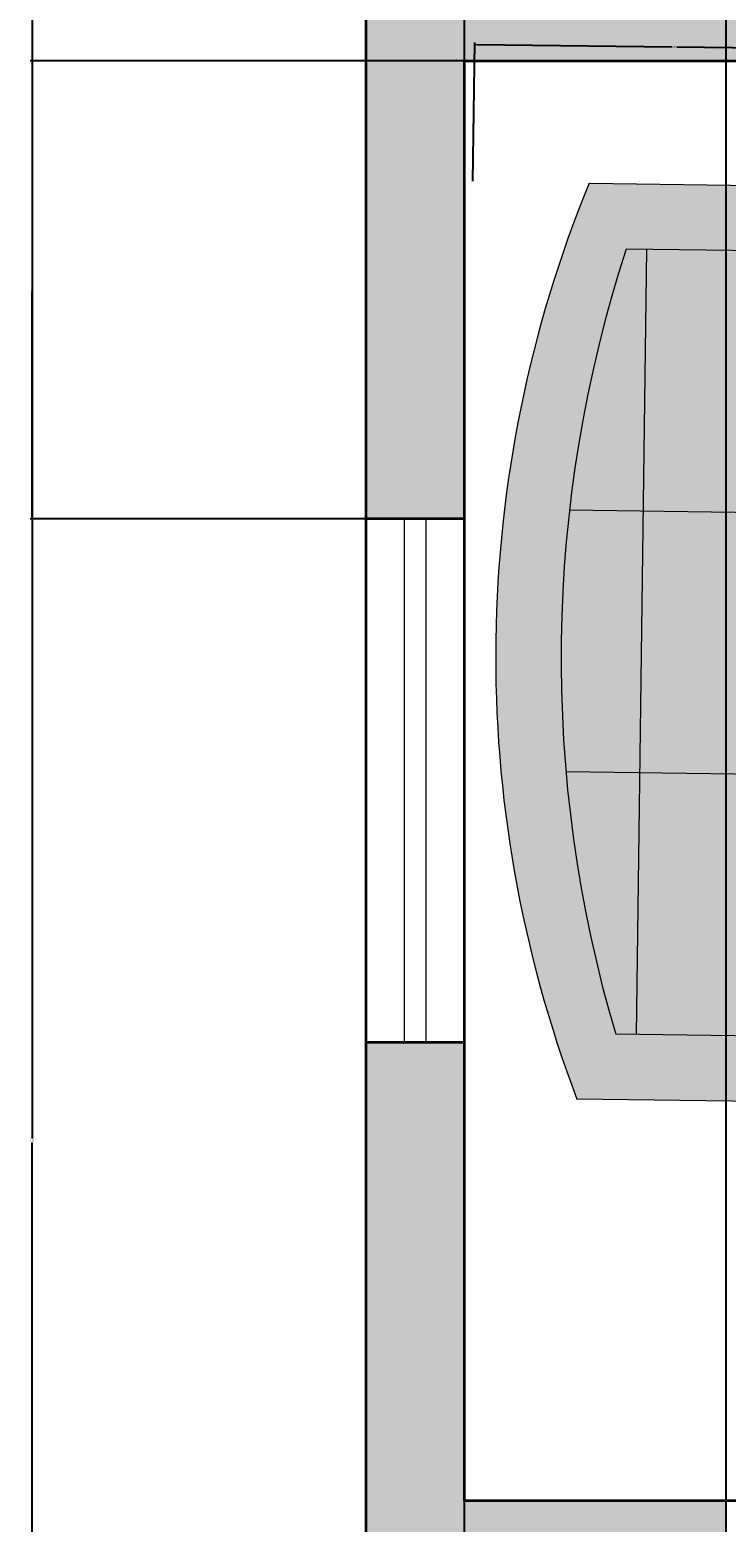
# Model space of a CAD drawing. Units: inches. Extents: x 1567 to 1964, y 1813 to 2447.
# Tile 7 of 28: x 1567 to 1630, y 2125 to 2262. Entities that reach past the tile are written whole.
import ezdxf

# ---------------------------------------------------------------- set-up
doc = ezdxf.new("R2010")
doc.units = ezdxf.units.IN
for name, color, linetype, lineweight in [('A-ANNO-DIMS', 2, 'Continuous', 18), ('A-FURN', 8, 'Continuous', 18), ('A-GLAZ', 4, 'Continuous', 18), ('A-WALL', 7, 'Continuous', 35)]:
    doc.layers.add(name, color=color, linetype=linetype, lineweight=lineweight)
doc.layers.add('A-FURN-PATT', color=252, linetype='Continuous', lineweight=13, true_color=0x939598)
doc.layers.add('A-WALL-PATT', color=251, linetype='Continuous', lineweight=13, true_color=0x636466)
doc.styles.get("Standard").update_dxf_attribs({"font": 'arial.ttf'})
doc.dimstyles.get("Standard").update_dxf_attribs({"dimtxt": 0.18, "dimasz": 0.18, "dimexe": 0.18, "dimexo": 0.0625, "dimgap": 0.09, "dimtad": 0, "dimtih": 1, "dimtoh": 1, "dimdec": 4, "dimzin": 0, "dimdsep": 46, "dimtxsty": 'Standard', "dimcen": 0.09, "dimadec": 0, "dimazin": 0, "dimtfac": 1, "dimtdec": 4, "dimtofl": 0, "dimtmove": 0, "dimatfit": 3, "dimfxl": 1, "dimtolj": 1, "dimtzin": 0, "dimarcsym": 0})

# ---------------------------------------------------------------- blocks, each defined once
blk = doc.blocks.new('Sofa - Roundback 7 ft.')
for p, q in [((-12.00002, -32.4421), (-12.00003, -6.5971)), ((11.99997, -32.4421), (11.99998, -6.5971)), ((-36.000027, -34), (-36.000027, -11.4696)), ((35.99998, -34), (35.99998, -11.4696)), ((-35.999844, -13.3819), (35.9998, -13.3819)), ((-36.000027, -32.4421), (35.99998, -32.4421))]:
    blk.add_line(p, q)
for points in [[(-36.000027, -34), (-42.000027, -34), (-42.000027, -8)], [(41.99998, -8), (41.99998, -34), (35.99998, -34)]]:
    blk.add_lwpolyline(points)
for centre, radius, start, end in [((0, -114.25), 114.25, 68.43141, 111.5686), ((-0.00001, -127.1968), 121.1968, 72.72033, 107.2797)]:
    blk.add_arc(centre, radius, start, end)
blk = doc.blocks.new('WINDOW-48IN')
for p, q in [((0, 2), (48, 2)), ((0, 0), (48, 0))]:
    blk.add_line(p, q)
blk = doc.blocks.new('*D24')
at = {"layer": 'A-ANNO-DIMS', "color": 0, "lineweight": -2, "transparency": 16777216}
for p, q in [((1607.2, 2248.27), (1607.37, 2260.99)), ((1607.54, 2260.81), (1625.48, 2260.57)), ((1643.85, 2260.32), (1625.92, 2260.56)), ((1643.86, 2247.79), (1644.03, 2260.5))]:
    blk.add_line(p, q, dxfattribs=at)
at = {"layer": 'A-ANNO-DIMS', "color": 0, "transparency": 16777216}
for points in [[(1607.54, 2260.84), (1607.54, 2260.78), (1607.36, 2260.81)], [(1643.85, 2260.35), (1643.85, 2260.29), (1644.03, 2260.32)]]:
    blk.add_solid(points, dxfattribs=at)
at = {"layer": 'Defpoints', "color": 0, "transparency": 16777216}
for p in [(1607.36, 2260.81), (1607.2, 2248.21), (1643.86, 2247.72)]:
    blk.add_point(p, dxfattribs=at)
at = {"layer": 'A-ANNO-DIMS', "color": 0, "transparency": 16777216, "insert": (1625.7, 2260.57), "char_height": 0.18, "attachment_point": 5}
blk.add_mtext('\\A1;37', dxfattribs=at)
blk = doc.blocks.new('*D41')
at = {"layer": 'A-ANNO-DIMS', "color": 0, "lineweight": -2, "transparency": 16777216}
for p, q in [((1597.37, 2416.29), (1566.6, 2416.29)), ((1566.78, 2416.11), (1566.78, 2160.47)), ((1566.78, 1904.47), (1566.78, 2160.11)), ((1601.37, 1904.29), (1566.6, 1904.29))]:
    blk.add_line(p, q, dxfattribs=at)
at = {"layer": 'A-ANNO-DIMS', "color": 0, "transparency": 16777216}
for points in [[(1566.75, 2416.11), (1566.81, 2416.11), (1566.78, 2416.29)], [(1566.75, 1904.47), (1566.81, 1904.47), (1566.78, 1904.29)]]:
    blk.add_solid(points, dxfattribs=at)
at = {"layer": 'Defpoints', "color": 0, "transparency": 16777216}
for p in [(1566.78, 2416.29), (1597.43, 2416.29), (1601.43, 1904.29)]:
    blk.add_point(p, dxfattribs=at)
at = {"layer": 'A-ANNO-DIMS', "color": 0, "transparency": 16777216, "insert": (1566.78, 2160.29), "char_height": 0.18, "attachment_point": 5}
blk.add_mtext('\\A1;512', dxfattribs=at)
blk = doc.blocks.new('*D50')
at = {"layer": 'A-ANNO-DIMS', "color": 0, "lineweight": -2, "transparency": 16777216}
for p, q in [((1606.37, 2259.29), (1566.6, 2259.29)), ((1566.78, 2259.11), (1566.78, 2238.47)), ((1566.78, 2217.47), (1566.78, 2238.11)), ((1597.37, 2217.29), (1566.6, 2217.29))]:
    blk.add_line(p, q, dxfattribs=at)
at = {"layer": 'A-ANNO-DIMS', "color": 0, "transparency": 16777216}
for points in [[(1566.75, 2259.11), (1566.81, 2259.11), (1566.78, 2259.29)], [(1566.75, 2217.47), (1566.81, 2217.47), (1566.78, 2217.29)]]:
    blk.add_solid(points, dxfattribs=at)
at = {"layer": 'Defpoints', "color": 0, "transparency": 16777216}
for p in [(1606.43, 2259.29), (1566.78, 2217.29), (1597.43, 2217.29)]:
    blk.add_point(p, dxfattribs=at)
at = {"layer": 'A-ANNO-DIMS', "color": 0, "transparency": 16777216, "insert": (1566.78, 2238.29), "char_height": 0.18, "attachment_point": 5}
blk.add_mtext('\\A1;42', dxfattribs=at)
blk = doc.blocks.new('*D53')
at = {"layer": 'A-ANNO-DIMS', "color": 0, "lineweight": -2, "transparency": 16777216}
for p, q in [((1606.43, 1913.35), (1606.43, 2447.12)), ((1606.61, 2446.94), (1618.21, 2446.94)), ((1630.25, 2446.94), (1618.65, 2446.94)), ((1630.43, 1913.35), (1630.43, 2447.12))]:
    blk.add_line(p, q, dxfattribs=at)
at = {"layer": 'A-ANNO-DIMS', "color": 0, "transparency": 16777216}
for points in [[(1606.61, 2446.97), (1606.61, 2446.91), (1606.43, 2446.94)], [(1630.25, 2446.97), (1630.25, 2446.91), (1630.43, 2446.94)]]:
    blk.add_solid(points, dxfattribs=at)
at = {"layer": 'Defpoints', "color": 0, "transparency": 16777216}
for p in [(1630.43, 2446.94), (1606.43, 1913.29), (1630.43, 1913.29)]:
    blk.add_point(p, dxfattribs=at)
at = {"layer": 'A-ANNO-DIMS', "color": 0, "transparency": 16777216, "insert": (1618.43, 2446.94), "char_height": 0.18, "attachment_point": 5}
blk.add_mtext('\\A1;24', dxfattribs=at)
blk = doc.blocks.new('*D56')
at = {"layer": 'A-ANNO-DIMS', "color": 0, "lineweight": -2, "transparency": 16777216}
for p, q in [((1606.43, 2127.35), (1606.43, 2447.12)), ((1606.61, 2446.94), (1618.21, 2446.94)), ((1630.25, 2446.94), (1618.65, 2446.94)), ((1630.43, 2127.35), (1630.43, 2447.12))]:
    blk.add_line(p, q, dxfattribs=at)
at = {"layer": 'A-ANNO-DIMS', "color": 0, "transparency": 16777216}
for points in [[(1606.61, 2446.97), (1606.61, 2446.91), (1606.43, 2446.94)], [(1630.25, 2446.97), (1630.25, 2446.91), (1630.43, 2446.94)]]:
    blk.add_solid(points, dxfattribs=at)
at = {"layer": 'Defpoints', "color": 0, "transparency": 16777216}
for p in [(1630.43, 2446.94), (1606.43, 2127.29), (1630.43, 2127.29)]:
    blk.add_point(p, dxfattribs=at)
at = {"layer": 'A-ANNO-DIMS', "color": 0, "transparency": 16777216, "insert": (1618.43, 2446.94), "char_height": 0.18, "attachment_point": 5}
blk.add_mtext('\\A1;24', dxfattribs=at)
blk = doc.blocks.new('*D57')
at = {"layer": 'A-ANNO-DIMS', "color": 0, "lineweight": -2, "transparency": 16777216}
for p, q in [((1630.43, 2127.35), (1630.43, 2447.12)), ((1630.61, 2446.94), (1654.21, 2446.94)), ((1678.25, 2446.94), (1654.65, 2446.94)), ((1678.43, 2127.35), (1678.43, 2447.12))]:
    blk.add_line(p, q, dxfattribs=at)
at = {"layer": 'A-ANNO-DIMS', "color": 0, "transparency": 16777216}
for points in [[(1630.61, 2446.97), (1630.61, 2446.91), (1630.43, 2446.94)], [(1678.25, 2446.97), (1678.25, 2446.91), (1678.43, 2446.94)]]:
    blk.add_solid(points, dxfattribs=at)
at = {"layer": 'Defpoints', "color": 0, "transparency": 16777216}
for p in [(1678.43, 2446.94), (1630.43, 2127.29), (1678.43, 2127.29)]:
    blk.add_point(p, dxfattribs=at)
at = {"layer": 'A-ANNO-DIMS', "color": 0, "transparency": 16777216, "insert": (1654.43, 2446.94), "char_height": 0.18, "attachment_point": 5}
blk.add_mtext('\\A1;48', dxfattribs=at)

msp = doc.modelspace()

# ---------------------------------------------------------------- hatches: boundary and pattern name
at = {"layer": 'A-FURN-PATT'}
h = msp.add_hatch(color=256, dxfattribs=at)
h.dxf.hatch_style = 1
h.paths.add_polyline_path([(1621.2532, 2242.0229), (1643.7811, 2241.7239), (1643.8607, 2247.7234), (1617.863, 2248.0685, 0.19047621), (1616.7481, 2164.0759), (1642.7458, 2163.7308), (1642.8254, 2169.7302), (1620.2975, 2170.0293, -0.15194781)])
h.paths.add_polyline_path([(1673.5306, 2249.6607), (1653.8509, 2249.6607), (1653.8509, 2248.5031, 0.11764706), (1673.5306, 2248.5031)])
h.paths.add_polyline_path([(1706.0889, 2249.6607), (1686.4092, 2249.6607), (1686.4092, 2248.5031, 0.11764706), (1706.0889, 2248.5031)])
h.paths.add_polyline_path([(1782.4511, 2227.4197), (1766.4511, 2227.4197), (1766.2949, 2226.4197), (1782.6074, 2226.4197)])
h.paths.add_polyline_path([(1810.4511, 2227.4197), (1794.4511, 2227.4197), (1794.2949, 2226.4197), (1810.6074, 2226.4197)])
h.paths.add_polyline_path([(1743.9511, 2208.076), (1742.9511, 2207.9197), (1742.9511, 2191.9197), (1743.9511, 2191.7635)])
h.paths.add_polyline_path([(1782.6074, 2173.4197), (1766.2949, 2173.4197), (1766.4511, 2172.4197), (1782.4511, 2172.4197)])
h.paths.add_polyline_path([(1810.6074, 2173.4197), (1794.2949, 2173.4197), (1794.4511, 2172.4197), (1810.4511, 2172.4197)])
h.paths.add_polyline_path([(1861.053, 2006.5071), (1845.8531, 2006.5071), (1861.053, 1991.3071)])
h.paths.add_polyline_path([(1905.853, 1993.7071), (1861.053, 1993.7071), (1861.053, 1991.3071), (1905.853, 1991.3071)])
h.paths.add_polyline_path([(1919.7245, 2257.29, 0.50000012), (1918.7245, 2258.29), (1901.7245, 2258.29, 0.50000012), (1900.7245, 2257.29), (1900.7245, 2253.29, 0.50000012), (1901.7245, 2252.29), (1918.7245, 2252.29, 0.50000012), (1919.7245, 2253.29)])
h.paths.add_polyline_path([(1875.9094, 2391.0204), (1875.9094, 2375.8204), (1891.1093, 2375.8204)], flags=17)
h.paths.add_polyline_path([(1891.1093, 2405.4204), (1831.1094, 2405.4204), (1831.1094, 2391.0204), (1839.1093, 2391.0204), (1839.1093, 2404.2204), (1859.9093, 2404.2204), (1859.9093, 2391.0204), (1862.3093, 2391.0204), (1862.3093, 2404.2204), (1883.1093, 2404.2204), (1883.1093, 2389.0204), (1877.9094, 2389.0204), (1891.1093, 2375.8204)])
h.paths.add_polyline_path([(1682.1402, 2390.0316), (1682.1402, 2374.8316), (1697.3402, 2374.8316)], flags=17)
h.paths.add_polyline_path([(1697.3402, 2404.4316), (1637.3402, 2404.4316), (1637.3402, 2390.0316), (1645.3402, 2390.0316), (1645.3402, 2403.2316), (1666.1402, 2403.2316), (1666.1402, 2390.0316), (1668.5402, 2390.0316), (1668.5402, 2403.2316), (1689.3402, 2403.2316), (1689.3402, 2388.0316), (1684.1402, 2388.0316), (1697.3402, 2374.8316)])
h = msp.add_hatch(color=256, dxfattribs=at)
h.dxf.hatch_style = 1
h.paths.add_polyline_path([(1642.2233, 2241.7446), (1623.1648, 2241.9976), (1622.8462, 2217.9997), (1641.9047, 2217.7467)])
h.paths.add_polyline_path([(1641.9047, 2217.7467), (1622.8462, 2217.9997), (1622.5277, 2194.0018), (1641.5862, 2193.7488)])
h.paths.add_polyline_path([(1641.5862, 2193.7488), (1622.5277, 2194.0018), (1622.2091, 2170.0039), (1641.2677, 2169.7509)])
h.paths.add_polyline_path([(1671.2154, 2243.8726, -0.23606798), (1673.5306, 2245.0302), (1673.5306, 2246.1879), (1653.8509, 2246.1879), (1653.8509, 2245.0302, -0.23606798), (1656.1662, 2243.8726), (1656.1662, 2233.4539, -0.23606798), (1653.8509, 2232.2963), (1653.8509, 2231.1387, 0.11764706), (1673.5306, 2231.1387), (1673.5306, 2232.2963, -0.23606798), (1671.2154, 2233.4539)])
h.paths.add_polyline_path([(1703.7736, 2243.8726, -0.23606798), (1706.0889, 2245.0302), (1706.0889, 2246.1879), (1686.4092, 2246.1879), (1686.4092, 2245.0302, -0.23606798), (1688.7245, 2243.8726), (1688.7245, 2233.4539, -0.23606798), (1686.4092, 2232.2963), (1686.4092, 2231.1387, 0.11764706), (1706.0889, 2231.1387), (1706.0889, 2232.2963, -0.23606798), (1703.7736, 2233.4539)])
h.paths.add_polyline_path([(1782.6855, 2225.9197), (1766.2168, 2225.9197), (1764.9668, 2217.9197), (1783.9356, 2217.9197)])
h.paths.add_polyline_path([(1810.6855, 2225.9197), (1794.2168, 2225.9197), (1792.9668, 2217.9197), (1811.9356, 2217.9197)])
h.paths.add_polyline_path([(1752.4511, 2209.4041), (1744.4511, 2208.1541), (1744.4511, 2191.6853), (1752.4511, 2190.4354)])
h.paths.add_polyline_path([(1783.9356, 2181.9197), (1764.9668, 2181.9197), (1766.2168, 2173.9197), (1782.6855, 2173.9197)])
h.paths.add_polyline_path([(1811.9356, 2181.9197), (1792.9668, 2181.9197), (1794.2168, 2173.9197), (1810.6855, 2173.9197)])
h.paths.add_polyline_path([(1832.4511, 2208.1541), (1824.4511, 2209.4041), (1824.4511, 2190.4354), (1832.4511, 2191.6853)])
h.paths.add_polyline_path([(1824.4511, 2194.4197), (1823.8775, 2194.266), (1823.2838, 2194.1743), (1822.6735, 2194.1363), (1822.0501, 2194.1437), (1821.4169, 2194.1882), (1820.7773, 2194.2615), (1820.1348, 2194.3554), (1819.4928, 2194.4614), (1818.8527, 2194.5726), (1818.2083, 2194.6873), (1817.5511, 2194.8049), (1816.873, 2194.9249), (1816.1656, 2195.0469), (1815.4205, 2195.1704), (1814.6296, 2195.2948), (1813.7845, 2195.4197), (1812.88, 2195.5442), (1811.9238, 2195.6658), (1810.9265, 2195.7815), (1809.899, 2195.8885), (1808.852, 2195.9837), (1807.7962, 2196.0643), (1806.7423, 2196.1273), (1805.7011, 2196.1697), (1804.6806, 2196.1896), (1803.6777, 2196.188), (1802.6865, 2196.1668), (1801.7011, 2196.1281), (1800.7158, 2196.0737), (1799.7245, 2196.0057), (1798.7216, 2195.9259), (1797.7011, 2195.8364), (1796.6564, 2195.7387), (1795.5781, 2195.6333), (1794.4557, 2195.52), (1793.2792, 2195.3989), (1792.0383, 2195.27), (1790.7226, 2195.1333), (1789.3219, 2194.9887), (1787.8261, 2194.8364), (1786.1882, 2194.6764), (1784.2148, 2194.5096), (1781.6759, 2194.3369), (1778.3417, 2194.1593), (1773.9821, 2193.9778), (1768.3671, 2193.7934), (1761.2668, 2193.6071), (1752.4511, 2193.4197), (1752.4511, 2189.9197), (1762.0489, 2190.1067), (1769.9836, 2190.2908), (1776.4672, 2190.469), (1781.7115, 2190.6385), (1785.9285, 2190.7962), (1789.33, 2190.9393), (1792.128, 2191.0648), (1794.5344, 2191.1697), (1796.7278, 2191.2521), (1798.7532, 2191.313), (1800.6223, 2191.3543), (1802.3469, 2191.3781), (1803.9387, 2191.3862), (1805.4094, 2191.3807), (1806.7708, 2191.3634), (1808.0345, 2191.3364), (1809.2127, 2191.3013), (1810.3196, 2191.2589), (1811.3699, 2191.2097), (1812.3782, 2191.1541), (1813.3592, 2191.0927), (1814.3274, 2191.0259), (1815.2976, 2190.9542), (1816.2845, 2190.8781), (1817.2985, 2190.7986), (1818.3339, 2190.7186), (1819.3811, 2190.6415), (1820.4303, 2190.5708), (1821.4716, 2190.5098), (1822.4954, 2190.4621), (1823.4918, 2190.4309), (1824.3581, 2190.4208), (1824.4511, 2190.4354)])
h.paths.add_polyline_path([(1874.6531, 1991.3071), (1861.053, 1991.3071), (1859.053, 1993.3071), (1853.8531, 1993.3071), (1853.8531, 1978.1071), (1874.6531, 1978.1071)], flags=17)
h.paths.add_polyline_path([(1897.8531, 1991.3071), (1877.0531, 1991.3071), (1877.0531, 1978.1071), (1897.8531, 1978.1071)], flags=17)
h.paths.add_polyline_path([(1853.8531, 1993.3071), (1859.053, 1993.3071), (1845.8531, 2006.5071), (1845.8531, 1976.9071), (1905.853, 1976.9071), (1905.853, 1991.3071), (1897.8531, 1991.3071), (1897.8531, 1978.1071), (1877.0531, 1978.1071), (1877.0531, 1991.3071), (1874.6531, 1991.3071), (1874.6531, 1978.1071), (1853.8531, 1978.1071)])
h.paths.add_polyline_path([(1920.7245, 2259.29), (1899.7245, 2259.29), (1899.7245, 2251.29), (1920.7245, 2251.29)])
h.paths.add_polyline_path([(1918.7245, 2252.29, 0.50000012), (1919.7245, 2253.29), (1919.7245, 2257.29, 0.50000012), (1918.7245, 2258.29), (1901.7245, 2258.29, 0.50000012), (1900.7245, 2257.29), (1900.7245, 2253.29, 0.50000012), (1901.7245, 2252.29)], flags=16)
h.paths.add_polyline_path([(1843.2327, 2065.967), (1919.26, 2065.967), (1919.26, 2095.8187), (1843.2327, 2095.8187)], flags=9)
h = msp.add_hatch(color=256, dxfattribs=at)
h.dxf.hatch_style = 1
h.paths.add_polyline_path([(1622.8462, 2217.9997), (1616.0605, 2218.0897, 0.04962821), (1615.7419, 2194.0919), (1622.5277, 2194.0018)])
h.paths.add_polyline_path([(1623.1648, 2241.9976), (1621.2532, 2242.0229, 0.05064665), (1616.0605, 2218.0897), (1622.8462, 2217.9997)])
h.paths.add_polyline_path([(1622.5277, 2194.0018), (1615.7419, 2194.0919, 0.05064665), (1620.2975, 2170.0293), (1622.2091, 2170.0039)])
h.paths.add_polyline_path([(1656.1662, 2243.8726, 0.5), (1651.5357, 2243.8726), (1651.5357, 2233.4539, 0.5), (1656.1662, 2233.4539)])
h.paths.add_polyline_path([(1675.8459, 2243.8726, 0.5), (1671.2154, 2243.8726), (1671.2154, 2233.4539, 0.5), (1675.8459, 2233.4539)])
h.paths.add_polyline_path([(1688.7245, 2243.8726, 0.5), (1684.094, 2243.8726), (1684.094, 2233.4539, 0.5), (1688.7245, 2233.4539)])
h.paths.add_polyline_path([(1708.4042, 2243.8726, 0.5), (1703.7736, 2243.8726), (1703.7736, 2233.4539, 0.5), (1708.4042, 2233.4539)])
at = {"layer": 'A-WALL-PATT'}
h = msp.add_hatch(color=256, dxfattribs=at)
h.dxf.hatch_style = 1
h.paths.add_polyline_path([(1606.4295, 2407.29), (1654.4295, 2407.29), (1654.4295, 2416.29), (1597.4295, 2416.29), (1597.4295, 2217.29), (1606.4295, 2217.29), (1606.4295, 2259.29), (1738.4295, 2259.29), (1738.4295, 2247.29), (1742.4295, 2247.29), (1742.4295, 2259.29), (1742.4295, 2272.29), (1738.4295, 2272.29), (1738.4295, 2263.29), (1606.4295, 2263.29)])
h.paths.add_polyline_path([(1753.4295, 2416.29), (1690.4295, 2416.29), (1690.4295, 2407.29), (1738.4295, 2407.29), (1738.4295, 2308.29), (1742.4295, 2308.29), (1742.4295, 2331.29), (1746.9295, 2331.29), (1746.9295, 2335.29), (1742.4295, 2335.29), (1742.4295, 2407.29), (1753.4295, 2407.29)])
h.paths.add_polyline_path([(1840.4295, 2416.29), (1777.4295, 2416.29), (1777.4295, 2407.29), (1788.4295, 2407.29), (1788.4295, 2335.29), (1776.9295, 2335.29), (1776.9295, 2331.29), (1788.4295, 2331.29), (1788.4295, 2308.29), (1792.4295, 2308.29), (1792.4295, 2407.29), (1840.4295, 2407.29)])
h.paths.add_polyline_path([(1933.4295, 2416.29), (1876.4295, 2416.29), (1876.4295, 2407.29), (1924.4295, 2407.29), (1924.4295, 2263.29), (1792.4295, 2263.29), (1792.4295, 2272.29), (1788.4295, 2272.29), (1788.4295, 2259.29), (1872.4295, 2259.29), (1872.4295, 2171.29), (1880.9295, 2171.29), (1880.9295, 2175.29), (1876.4295, 2175.29), (1876.4295, 2259.29), (1924.4295, 2259.29), (1924.4295, 2229.29), (1933.4295, 2229.29)])
h.paths.add_polyline_path([(1933.4295, 2205.29), (1924.4295, 2205.29), (1924.4295, 2175.29), (1910.9295, 2175.29), (1910.9295, 2171.29), (1924.4295, 2171.29), (1924.4295, 2127.29), (1844.4295, 2127.29), (1844.4295, 2123.29), (1924.4295, 2123.29), (1924.4295, 2063.29), (1933.4295, 2063.29)])
h.paths.add_polyline_path([(1799.4295, 2123.29), (1808.4295, 2123.29), (1808.4295, 2127.29), (1781.4295, 2127.29), (1781.4295, 2123.29), (1795.4295, 2123.29), (1795.4295, 1964.29), (1711.4295, 1964.29), (1711.4295, 2123.29), (1751.4295, 2123.29), (1751.4295, 2127.29), (1742.4295, 2127.29), (1742.4295, 2139.29), (1738.4295, 2139.29), (1738.4295, 2127.29), (1678.4295, 2127.29), (1678.4295, 2123.29), (1702.4295, 2123.29), (1702.4295, 1913.29), (1678.4295, 1913.29), (1678.4295, 1904.29), (1711.4295, 1904.29), (1711.4295, 1960.29), (1795.4295, 1960.29), (1795.4295, 1906.69), (1929.4295, 1906.69), (1929.4295, 1848.29), (1601.4295, 1848.29), (1601.4295, 1904.29), (1630.4295, 1904.29), (1630.4295, 1913.29), (1606.4295, 1913.29), (1606.4295, 2123.29), (1630.4295, 2123.29), (1630.4295, 2127.29), (1606.4295, 2127.29), (1606.4295, 2169.29), (1597.4295, 2169.29), (1597.4295, 1844.29), (1933.4295, 1844.29), (1933.4295, 2027.29), (1924.4295, 2027.29), (1924.4295, 1967.29), (1833.9295, 1967.29), (1833.9295, 1963.29), (1924.4295, 1963.29), (1924.4295, 1910.69), (1799.4295, 1910.69), (1799.4295, 1963.29), (1803.9295, 1963.29), (1803.9295, 1967.29), (1799.4295, 1967.29)])

# ---------------------------------------------------------------- linework, layer by layer
at = {"layer": 'A-WALL'}
for p, q in [((1597.4295, 1844.29), (1597.4295, 2416.29)), ((1606.4295, 2259.29), (1738.4295, 2259.29)), ((1606.4295, 2127.29), (1606.4295, 2259.29)), ((1606.4295, 2217.29), (1597.4295, 2217.29)), ((1606.4295, 2169.29), (1597.4295, 2169.29)), ((1606.4295, 2127.29), (1631.4295, 2127.29))]:
    msp.add_line(p, q, dxfattribs=at)

# ---------------------------------------------------------------- block references
at = {"layer": 'A-FURN', "rotation": 89.2395118843373}
msp.add_blockref('Sofa - Roundback 7 ft.', (1609.3062, 2206.1784), dxfattribs=at)
at = {"layer": 'A-GLAZ', "rotation": 90.00000000000003}
msp.add_blockref('WINDOW-48IN', (1602.9295, 2169.2905), dxfattribs=at)

# ---------------------------------------------------------------- dimensions: what is measured, and where the dimension line sits
at = {"layer": 'A-ANNO-DIMS'}
for base, p1, p2, picture, middle in [((1630.4295, 2446.94), (1606.4295, 1913.29), (1630.4295, 1913.29), '*D53', (1618.4295, 2446.94)), ((1630.4295, 2446.94), (1606.4295, 2127.29), (1630.4295, 2127.29), '*D56', (1618.4295, 2446.94)), ((1678.4295, 2446.94), (1630.4295, 2127.29), (1678.4295, 2127.29), '*D57', (1654.4295, 2446.94))]:
    dim = msp.add_linear_dim(base=base, p1=p1, p2=p2, dimstyle='Standard', override={"dimdec": 0, "dimlfac": 1, "dimrnd": 0, "dimzin": 0, "dimdsep": 46, "dimlunit": 2}, dxfattribs=at)
    dim.commit()
    dim.dimension.update_dxf_attribs({"geometry": picture, "text_midpoint": middle})
for base, p1, p2, angle, picture, middle in [((1566.7795, 2416.29), (1601.4295, 1904.29), (1597.4295, 2416.29), 90, '*D41', (1566.7795, 2160.29)), ((1607.3645, 2260.8089), (1643.8607, 2247.7234), (1607.1972, 2248.21), 179.239512, '*D24', (1625.6962, 2260.5656)), ((1566.7795, 2217.29), (1606.4295, 2259.29), (1597.4295, 2217.29), 90, '*D50', (1566.7795, 2238.29))]:
    dim = msp.add_linear_dim(base=base, p1=p1, p2=p2, angle=angle, dimstyle='Standard', override={"dimdec": 0, "dimlfac": 1, "dimrnd": 0, "dimzin": 0, "dimdsep": 46, "dimlunit": 2}, dxfattribs=at)
    dim.commit()
    dim.dimension.update_dxf_attribs({"geometry": picture, "text_midpoint": middle})

doc.saveas('drawing.dxf')
